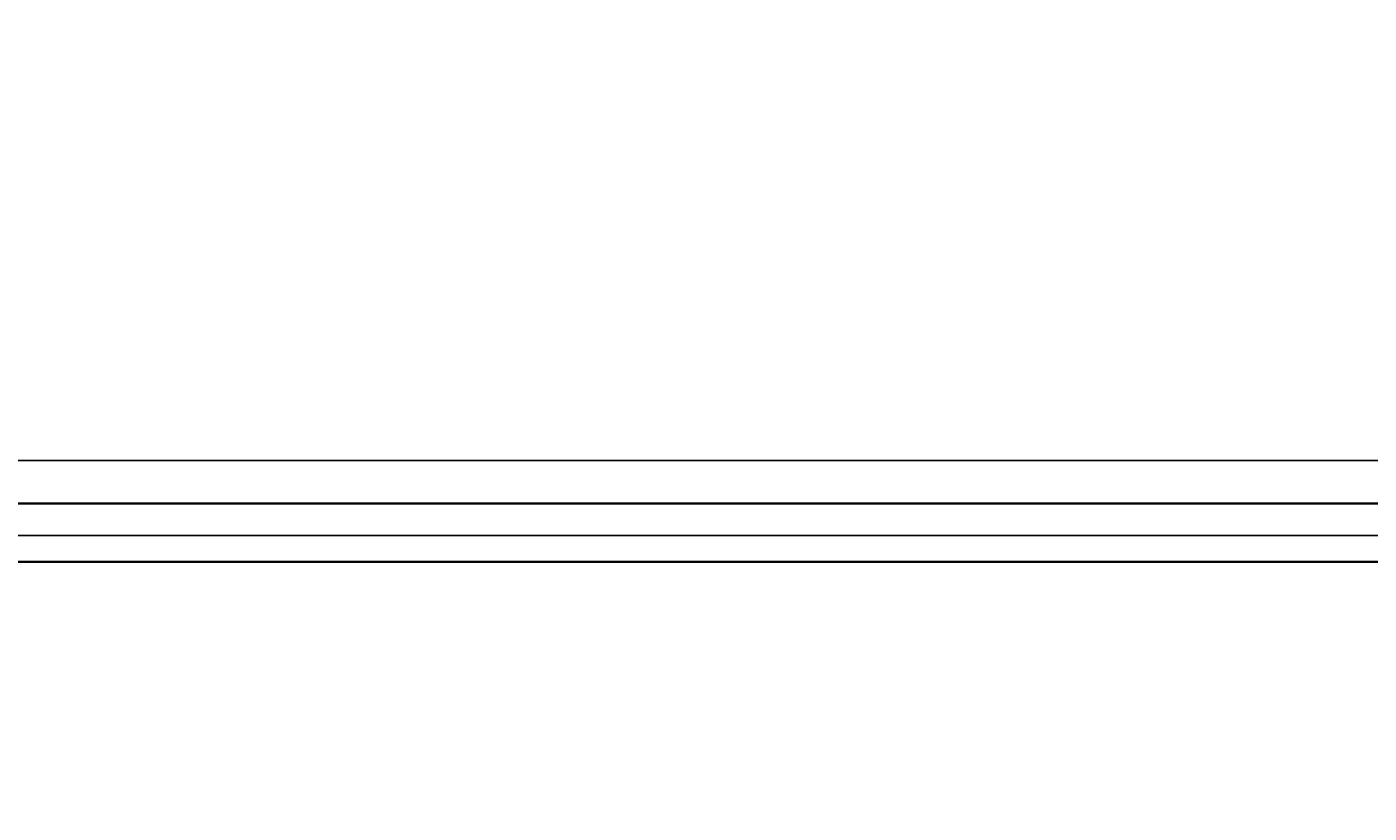
# Model space of a CAD drawing. Units: inches. Extents: x -6 to 289, y -8 to 323.
# Tile 9 of 107: x 48 to 102, y 37 to 68. Entities that reach past the tile are written whole.
import ezdxf

# ---------------------------------------------------------------- set-up
doc = ezdxf.new("R2010")
doc.units = ezdxf.units.IN
doc.header["$MEASUREMENT"] = 0
doc.layers.add('A-ANNO-DIMS', color=2, linetype='Continuous', lineweight=18)
doc.layers.add('A-ELEV', color=7, linetype='Continuous', lineweight=35)
doc.styles.get("Standard").update_dxf_attribs({"font": 'arial.ttf'})
doc.dimstyles.get("Standard").update_dxf_attribs({"dimtxt": 0.18, "dimasz": 0.18, "dimexe": 0.18, "dimexo": 0.0625, "dimgap": 0.09, "dimtad": 0, "dimtih": 1, "dimtoh": 1, "dimdec": 4, "dimzin": 0, "dimdsep": 46, "dimtxsty": 'Standard', "dimcen": 0.09, "dimadec": 0, "dimazin": 0, "dimtfac": 1, "dimtdec": 4, "dimtofl": 0, "dimtmove": 0, "dimatfit": 3, "dimfxl": 1, "dimtolj": 1, "dimtzin": 0, "dimarcsym": 0})

# ---------------------------------------------------------------- blocks, each defined once
blk = doc.blocks.new('*D16')
at = {"layer": 'A-ANNO-DIMS', "color": 0, "lineweight": -2, "transparency": 16777216}
for p, q in [((9.943, 68.37), (9.943, -8.391)), ((272.973, 68.37), (272.973, -8.391)), ((10.123, -8.211), (140.993, -8.211)), ((272.793, -8.211), (141.923, -8.211))]:
    blk.add_line(p, q, dxfattribs=at)
at = {"layer": 'A-ANNO-DIMS', "color": 0, "transparency": 16777216}
for points in [[(10.123, -8.181), (10.123, -8.241), (9.943, -8.211)], [(272.793, -8.181), (272.793, -8.241), (272.973, -8.211)]]:
    blk.add_solid(points, dxfattribs=at)
at = {"layer": 'Defpoints', "color": 0, "transparency": 16777216}
for p in [(9.943, 68.432), (272.973, 68.432), (272.973, -8.211)]:
    blk.add_point(p, dxfattribs=at)
at = {"layer": 'A-ANNO-DIMS', "color": 0, "transparency": 16777216, "insert": (141.458, -8.211), "char_height": 0.18, "attachment_point": 5}
blk.add_mtext('\\A1;263.03', dxfattribs=at)
blk = doc.blocks.new('*D84')
at = {"layer": 'A-ANNO-DIMS', "color": 0, "lineweight": -2, "transparency": 16777216}
for p, q in [((123.945, 48.085), (-5.737, 48.085)), ((-5.557, 47.905), (-5.557, 29.369)), ((-5.557, 10.469), (-5.557, 29.005)), ((123.945, 10.289), (-5.737, 10.289))]:
    blk.add_line(p, q, dxfattribs=at)
at = {"layer": 'A-ANNO-DIMS', "color": 0, "transparency": 16777216}
for points in [[(-5.587, 47.905), (-5.527, 47.905), (-5.557, 48.085)], [(-5.587, 10.469), (-5.527, 10.469), (-5.557, 10.289)]]:
    blk.add_solid(points, dxfattribs=at)
at = {"layer": 'Defpoints', "color": 0, "transparency": 16777216}
for p in [(-5.557, 48.085), (124.008, 48.085), (124.008, 10.289)]:
    blk.add_point(p, dxfattribs=at)
at = {"layer": 'A-ANNO-DIMS', "color": 0, "transparency": 16777216, "insert": (-5.557, 29.187), "char_height": 0.18, "attachment_point": 5}
blk.add_mtext('\\A1;37.8', dxfattribs=at)
blk = doc.blocks.new('*D85')
at = {"layer": 'A-ANNO-DIMS', "color": 0, "lineweight": -2, "transparency": 16777216}
for p, q in [((120.945, 51.085), (-5.737, 51.085)), ((-5.557, 50.905), (-5.557, 49.767)), ((-5.557, 48.265), (-5.557, 49.403)), ((123.945, 48.085), (-5.737, 48.085))]:
    blk.add_line(p, q, dxfattribs=at)
at = {"layer": 'A-ANNO-DIMS', "color": 0, "transparency": 16777216}
for points in [[(-5.587, 50.905), (-5.527, 50.905), (-5.557, 51.085)], [(-5.587, 48.265), (-5.527, 48.265), (-5.557, 48.085)]]:
    blk.add_solid(points, dxfattribs=at)
at = {"layer": 'Defpoints', "color": 0, "transparency": 16777216}
for p in [(-5.557, 51.085), (121.008, 51.085), (124.008, 48.085)]:
    blk.add_point(p, dxfattribs=at)
at = {"layer": 'A-ANNO-DIMS', "color": 0, "transparency": 16777216, "insert": (-5.557, 49.585), "char_height": 0.18, "attachment_point": 5}
blk.add_mtext('\\A1;3', dxfattribs=at)
blk = doc.blocks.new('*D86')
at = {"layer": 'A-ANNO-DIMS', "color": 0, "lineweight": -2, "transparency": 16777216}
for p, q in [((166.233, 75.971), (-5.737, 75.971)), ((-5.557, 75.791), (-5.557, 63.71)), ((-5.557, 51.265), (-5.557, 63.346)), ((120.945, 51.085), (-5.737, 51.085))]:
    blk.add_line(p, q, dxfattribs=at)
at = {"layer": 'A-ANNO-DIMS', "color": 0, "transparency": 16777216}
for points in [[(-5.587, 75.791), (-5.527, 75.791), (-5.557, 75.971)], [(-5.587, 51.265), (-5.527, 51.265), (-5.557, 51.085)]]:
    blk.add_solid(points, dxfattribs=at)
at = {"layer": 'Defpoints', "color": 0, "transparency": 16777216}
for p in [(-5.557, 75.971), (166.296, 75.971), (121.008, 51.085)]:
    blk.add_point(p, dxfattribs=at)
at = {"layer": 'A-ANNO-DIMS', "color": 0, "transparency": 16777216, "insert": (-5.557, 63.528), "char_height": 0.18, "attachment_point": 5}
blk.add_mtext('\\A1;24.886', dxfattribs=at)

msp = doc.modelspace()

# ---------------------------------------------------------------- linework, layer by layer
at = {"layer": 'A-ELEV'}
for points in [[(24.317, 49.3604), (108.6602, 49.3604), (108.6602, 7.2888), (24.317, 7.2888)], [(24.317, 49.3604), (108.6602, 49.3604), (108.6602, 47.0304), (24.317, 47.0304)]]:
    msp.add_lwpolyline(points, close=True, dxfattribs=at)

# ---------------------------------------------------------------- dimensions: what is measured, and where the dimension line sits
at = {"layer": 'A-ANNO-DIMS'}
for base, p1, p2, override, picture, middle in [((-5.557, 75.97064), (121.00798, 51.08513), (166.29599, 75.97064), {"dimdec": 3, "dimlfac": 1, "dimrnd": 0, "dimzin": 0, "dimdsep": 46, "dimlunit": 2}, '*D86', (-5.557, 63.52788)), ((-5.557, 51.0851), (124.008, 48.0851), (121.008, 51.0851), {"dimdec": 0, "dimlfac": 1, "dimrnd": 0, "dimzin": 0, "dimdsep": 46, "dimlunit": 2}, '*D85', (-5.557, 49.5851)), ((-5.557, 48.0851), (124.008, 10.2888), (124.008, 48.0851), {"dimdec": 1, "dimlfac": 1, "dimrnd": 0, "dimzin": 0, "dimdsep": 46, "dimlunit": 2}, '*D84', (-5.557, 29.187))]:
    dim = msp.add_linear_dim(base=base, p1=p1, p2=p2, angle=90, dimstyle='Standard', override=override, dxfattribs=at)
    dim.commit()
    dim.dimension.update_dxf_attribs({"geometry": picture, "text_midpoint": middle})
dim = msp.add_linear_dim(base=(272.9733, -8.2112), p1=(9.943, 68.4322), p2=(272.9733, 68.4322), dimstyle='Standard', override={"dimdec": 2, "dimlfac": 1, "dimrnd": 0, "dimzin": 0, "dimdsep": 46, "dimlunit": 2}, dxfattribs=at)
dim.commit()
dim.dimension.update_dxf_attribs({"geometry": '*D16', "text_midpoint": (141.4581, -8.2112)})

doc.saveas('drawing.dxf')
